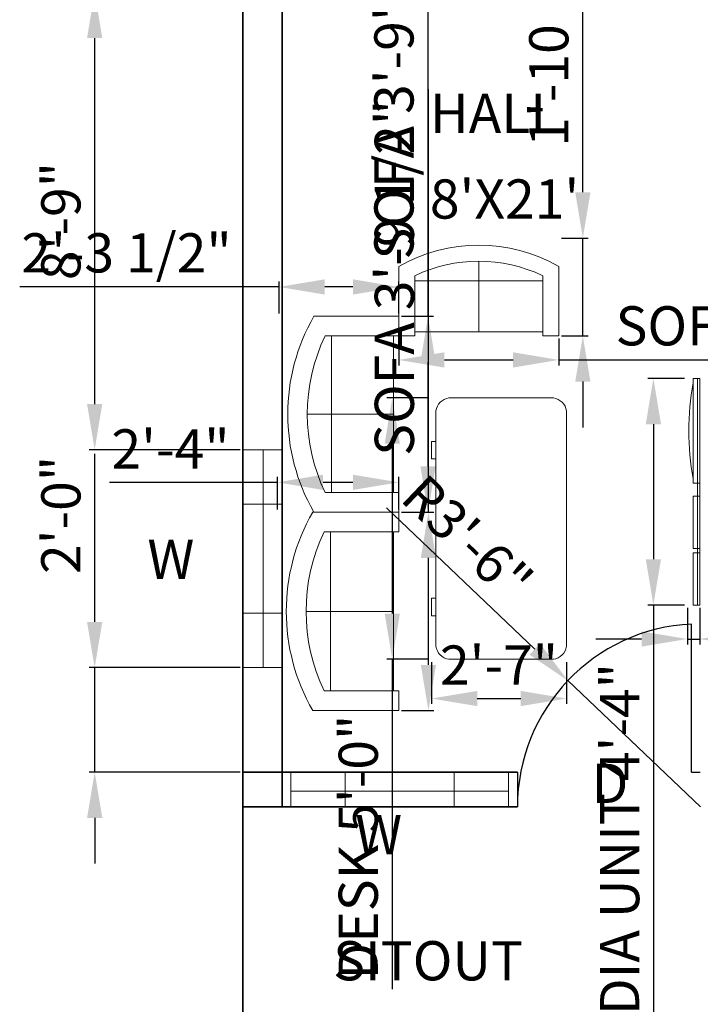
# Model space of a CAD drawing. Units: inches. Extents: x 1956 to 4770, y 1551 to 2596.
# Tile 3 of 10: x 2207 to 2363, y 1865 to 2091. Entities that reach past the tile are written whole.
import ezdxf

# ---------------------------------------------------------------- set-up
doc = ezdxf.new("R2010")
doc.units = ezdxf.units.IN
for name, color, linetype, lineweight in [('A-ANNO-DIMS', 2, 'Continuous', 18), ('A-ANNO-TEXT', 7, 'Continuous', 18), ('A-AREA-IDEN', 7, 'Continuous', 18), ('A-DOOR', 3, 'Continuous', 25), ('A-FURN', 8, 'Continuous', 18), ('A-GLAZ', 4, 'Continuous', 18), ('A-WALL', 7, 'Continuous', 35)]:
    doc.layers.add(name, color=color, linetype=linetype, lineweight=lineweight)
doc.styles.get("Standard").update_dxf_attribs({"font": 'arial.ttf'})
doc.dimstyles.new('ISO-25', dxfattribs={"dimtxt": 9, "dimasz": 10.5, "dimexe": 1.25, "dimexo": 0.625, "dimgap": 2, "dimtad": 1, "dimdec": 1, "dimlunit": 4, "dimtxsty": 'Standard', "dimcen": 2.5, "dimadec": 0, "dimazin": 0, "dimtfac": 1, "dimtdec": 1, "dimtmove": 0, "dimatfit": 3, "dimfxl": 1, "dimarcsym": 0})

# ---------------------------------------------------------------- blocks, each defined once
blk = doc.blocks.new('Sofa - Roundback Loveseat 5 ft.')
for p, q in [((0, -32.44198), (0, -5.99998)), ((-24, -33.99998), (-24, -11.46958)), ((24.00004, -33.99998), (24.00004, -11.46958)), ((-23.9998, -13.38178), (23.99986, -13.38178)), ((-24, -32.44198), (24.00004, -32.44198))]:
    blk.add_line(p, q)
for points in [[(-24, -33.99998), (-30, -33.99998), (-30, -7.99998)], [(30.00004, -7.99998), (30.00004, -33.99998), (24.00004, -33.99998)]]:
    blk.add_lwpolyline(points)
for centre, radius, start, end in [((0, -60.24998), 60.24998, 60.13715, 119.8628), ((0, -61.38438), 55.38444, 64.32083, 115.6792)]:
    blk.add_arc(centre, radius, start, end)
blk = doc.blocks.new('Desk - 30 x 60 in.')
for p, q in [((-26.999995, 0), (26.999995, 0)), ((-29.999995, -27), (-29.999995, -3)), ((29.999995, -3), (29.999995, -27)), ((26.999995, -30), (-26.999995, -30)), ((-20.000005, -30), (-20.000005, -31)), ((-20.000005, -31), (-16.000005, -31)), ((-16.000005, -31), (-16.000005, -30)), ((15.999995, -31), (15.999995, -30)), ((19.999995, -31), (15.999995, -31)), ((19.999995, -30), (19.999995, -31))]:
    blk.add_line(p, q)
for centre, start, end in [((-26.499995, -3.5), 98.1301, 171.8699), ((26.499995, -3.5), 8.130102, 81.8699), ((-26.499995, -26.5), 188.1301, 261.8699), ((26.499995, -26.5), 278.1301, 351.8699)]:
    blk.add_arc(centre, 3.535534, start, end)
blk = doc.blocks.new('Entertainment Center')
for p, q in [((-12, -20), (-12, -18.5)), ((40, -18.5), (-12, -18.5)), ((40, -19), (-12, -19)), ((12, -20), (-12, -20)), ((12, -18.5), (12, -20)), ((15, -20), (15, -18.5)), ((27, -20), (15, -20)), ((27, -18.5), (27, -20)), ((28, -20), (28, -18.5)), ((40, -20), (28, -20)), ((40, -18.5), (40, -20))]:
    blk.add_line(p, q)
blk.add_arc((0, 40), 61, 259.6111, 280.3889)
blk = doc.blocks.new('WIN-50IN-WALL9')
for p, q in [((0, 50), (9, 50)), ((4.6, 50), (4.6, 0)), ((0, 37.5), (9, 37.5)), ((9, 12.5), (0, 12.5)), ((9, 0), (1, 0)), ((0, 0), (9, 0))]:
    blk.add_line(p, q)
blk = doc.blocks.new('WIN-50IN-WALL8')
for p, q in [((0, 0), (0, 8)), ((12.5, 0), (12.5, 8)), ((37.5, 8), (37.5, 0)), ((50, 8), (50, 0)), ((0, 3.6), (50, 3.6))]:
    blk.add_line(p, q)
blk = doc.blocks.new('*D31')
at = {"layer": 'A-ANNO-DIMS', "color": 0, "lineweight": -2, "transparency": 16777216}
for p, q in [((2294, 2017.6), (2294, 2011.46)), ((2330.76, 2017.6), (2330.76, 2011.46)), ((2304.5, 2012.71), (2320.26, 2012.71)), ((2330.76, 2012.71), (2406.87, 2012.71))]:
    blk.add_line(p, q, dxfattribs=at)
at = {"layer": 'A-ANNO-DIMS', "color": 0, "transparency": 16777216}
for points in [[(2304.5, 2014.46), (2304.5, 2010.96), (2294, 2012.71)], [(2320.26, 2014.46), (2320.26, 2010.96), (2330.76, 2012.71)]]:
    blk.add_solid(points, dxfattribs=at)
at = {"layer": 'Defpoints', "color": 0, "transparency": 16777216}
for p in [(2294, 2018.23), (2330.76, 2018.23), (2330.76, 2012.71)]:
    blk.add_point(p, dxfattribs=at)
at = {"layer": 'A-ANNO-DIMS', "color": 0, "transparency": 16777216, "insert": (2374.07, 2019.37), "char_height": 9, "attachment_point": 5}
blk.add_mtext('SOFA 3\'-1"', dxfattribs=at)
blk = doc.blocks.new('*D32')
at = {"layer": 'A-ANNO-DIMS', "color": 0, "lineweight": -2, "transparency": 16777216}
for p, q in [((2336.28, 2051.19), (2336.28, 2116.73)), ((2331.39, 2040.69), (2337.53, 2040.69)), ((2336.28, 2018.23), (2336.28, 2040.69)), ((2331.39, 2018.23), (2337.53, 2018.23)), ((2336.28, 2007.73), (2336.28, 1997.23))]:
    blk.add_line(p, q, dxfattribs=at)
at = {"layer": 'A-ANNO-DIMS', "color": 0, "transparency": 16777216}
for points in [[(2334.53, 2051.19), (2338.03, 2051.19), (2336.28, 2040.69)], [(2334.53, 2007.73), (2338.03, 2007.73), (2336.28, 2018.23)]]:
    blk.add_solid(points, dxfattribs=at)
at = {"layer": 'Defpoints', "color": 0, "transparency": 16777216}
for p in [(2330.76, 2040.69), (2336.28, 2040.69), (2330.76, 2018.23)]:
    blk.add_point(p, dxfattribs=at)
at = {"layer": 'A-ANNO-DIMS', "color": 0, "transparency": 16777216, "insert": (2329.63, 2089.21), "char_height": 9, "attachment_point": 5, "rotation": 90}
blk.add_mtext('1\'-10 1/2"', dxfattribs=at)
blk = doc.blocks.new('*D33')
at = {"layer": 'A-ANNO-DIMS', "color": 0, "lineweight": -2, "transparency": 16777216}
for p, q in [((2300.83, 1977.77), (2300.83, 2074.85)), ((2294.63, 1977.77), (2302.08, 1977.77)), ((2300.83, 1942.72), (2300.83, 1967.27)), ((2294.63, 1932.22), (2302.08, 1932.22))]:
    blk.add_line(p, q, dxfattribs=at)
at = {"layer": 'A-ANNO-DIMS', "color": 0, "transparency": 16777216}
for points in [[(2299.08, 1967.27), (2302.58, 1967.27), (2300.83, 1977.77)], [(2299.08, 1942.72), (2302.58, 1942.72), (2300.83, 1932.22)]]:
    blk.add_solid(points, dxfattribs=at)
at = {"layer": 'Defpoints', "color": 0, "transparency": 16777216}
for p in [(2294, 1977.77), (2300.83, 1977.77), (2294, 1932.22)]:
    blk.add_point(p, dxfattribs=at)
at = {"layer": 'A-ANNO-DIMS', "color": 0, "transparency": 16777216, "insert": (2294.17, 2031.56), "char_height": 9, "attachment_point": 5, "rotation": 90}
blk.add_mtext('SOFA 3\'-9 1/2"', dxfattribs=at)
blk = doc.blocks.new('*D34')
at = {"layer": 'A-ANNO-DIMS', "color": 0, "lineweight": -2, "transparency": 16777216}
for p, q in [((2266.16, 1984.61), (2227.58, 1984.61)), ((2266.16, 1978.4), (2266.16, 1985.86)), ((2283.5, 1984.61), (2276.66, 1984.61)), ((2294, 1978.4), (2294, 1985.86))]:
    blk.add_line(p, q, dxfattribs=at)
at = {"layer": 'A-ANNO-DIMS', "color": 0, "transparency": 16777216}
for points in [[(2276.66, 1986.36), (2276.66, 1982.86), (2266.16, 1984.61)], [(2283.5, 1986.36), (2283.5, 1982.86), (2294, 1984.61)]]:
    blk.add_solid(points, dxfattribs=at)
at = {"layer": 'Defpoints', "color": 0, "transparency": 16777216}
for p in [(2266.16, 1984.61), (2266.16, 1977.77), (2294, 1977.77)]:
    blk.add_point(p, dxfattribs=at)
at = {"layer": 'A-ANNO-DIMS', "color": 0, "transparency": 16777216, "insert": (2241.62, 1991.12), "char_height": 9, "attachment_point": 5}
blk.add_mtext('2\'-4"', dxfattribs=at)
blk = doc.blocks.new('*D35')
at = {"layer": 'A-ANNO-DIMS', "color": 0, "lineweight": -2, "transparency": 16777216}
for p, q in [((2300.74, 2022.72), (2300.74, 2098.83)), ((2294.63, 2022.72), (2301.99, 2022.72)), ((2300.74, 1988.27), (2300.74, 2012.22)), ((2294.63, 1977.77), (2301.99, 1977.77))]:
    blk.add_line(p, q, dxfattribs=at)
at = {"layer": 'A-ANNO-DIMS', "color": 0, "transparency": 16777216}
for points in [[(2298.99, 2012.22), (2302.49, 2012.22), (2300.74, 2022.72)], [(2298.99, 1988.27), (2302.49, 1988.27), (2300.74, 1977.77)]]:
    blk.add_solid(points, dxfattribs=at)
at = {"layer": 'Defpoints', "color": 0, "transparency": 16777216}
for p in [(2294, 2022.72), (2300.74, 2022.72), (2294, 1977.77)]:
    blk.add_point(p, dxfattribs=at)
at = {"layer": 'A-ANNO-DIMS', "color": 0, "transparency": 16777216, "insert": (2294.08, 2066.02), "char_height": 9, "attachment_point": 5, "rotation": 90}
blk.add_mtext('SOFA 3\'-9"', dxfattribs=at)
blk = doc.blocks.new('*D36')
at = {"layer": 'A-ANNO-DIMS', "color": 0, "lineweight": -2, "transparency": 16777216}
for p, q in [((2266.53, 2023.35), (2266.53, 2030.71)), ((2294, 2023.35), (2294, 2030.71)), ((2266.53, 2029.46), (2206.98, 2029.46)), ((2283.5, 2029.46), (2277.03, 2029.46))]:
    blk.add_line(p, q, dxfattribs=at)
at = {"layer": 'A-ANNO-DIMS', "color": 0, "transparency": 16777216}
for points in [[(2277.03, 2031.21), (2277.03, 2027.71), (2266.53, 2029.46)], [(2283.5, 2031.21), (2283.5, 2027.71), (2294, 2029.46)]]:
    blk.add_solid(points, dxfattribs=at)
at = {"layer": 'Defpoints', "color": 0, "transparency": 16777216}
for p in [(2266.53, 2029.46), (2266.53, 2022.72), (2294, 2022.72)]:
    blk.add_point(p, dxfattribs=at)
at = {"layer": 'A-ANNO-DIMS', "color": 0, "transparency": 16777216, "insert": (2231.51, 2036.12), "char_height": 9, "attachment_point": 5}
blk.add_mtext('2\'-3 1/2"', dxfattribs=at)
blk = doc.blocks.new('*D59')
at = {"layer": 'A-ANNO-DIMS', "color": 0, "lineweight": -2, "transparency": 16777216}
for p, q in [((2300.91, 2003.99), (2291.28, 2003.99)), ((2292.53, 1993.49), (2292.53, 1954.49)), ((2300.91, 1943.99), (2291.28, 1943.99)), ((2292.53, 1943.99), (2292.53, 1868.28))]:
    blk.add_line(p, q, dxfattribs=at)
at = {"layer": 'A-ANNO-DIMS', "color": 0, "transparency": 16777216}
for points in [[(2290.78, 1993.49), (2294.28, 1993.49), (2292.53, 2003.99)], [(2290.78, 1954.49), (2294.28, 1954.49), (2292.53, 1943.99)]]:
    blk.add_solid(points, dxfattribs=at)
at = {"layer": 'Defpoints', "color": 0, "transparency": 16777216}
for p in [(2301.53, 2003.99), (2292.53, 1943.99), (2301.53, 1943.99)]:
    blk.add_point(p, dxfattribs=at)
at = {"layer": 'A-ANNO-DIMS', "color": 0, "transparency": 16777216, "insert": (2285.88, 1900.88), "char_height": 9, "attachment_point": 5, "rotation": 90}
blk.add_mtext('DESK 5\'-0"', dxfattribs=at)
blk = doc.blocks.new('*D60')
at = {"layer": 'A-ANNO-DIMS', "color": 0, "lineweight": -2, "transparency": 16777216}
for p, q in [((2301.53, 1943.36), (2301.53, 1933.74)), ((2332.53, 1943.36), (2332.53, 1933.74)), ((2312.03, 1934.99), (2322.03, 1934.99))]:
    blk.add_line(p, q, dxfattribs=at)
at = {"layer": 'A-ANNO-DIMS', "color": 0, "transparency": 16777216}
for points in [[(2312.03, 1936.74), (2312.03, 1933.24), (2301.53, 1934.99)], [(2322.03, 1936.74), (2322.03, 1933.24), (2332.53, 1934.99)]]:
    blk.add_solid(points, dxfattribs=at)
at = {"layer": 'Defpoints', "color": 0, "transparency": 16777216}
for p in [(2301.53, 1943.99), (2332.53, 1943.99), (2332.53, 1934.99)]:
    blk.add_point(p, dxfattribs=at)
at = {"layer": 'A-ANNO-DIMS', "color": 0, "transparency": 16777216, "insert": (2317.03, 1941.5), "char_height": 9, "attachment_point": 5}
blk.add_mtext('2\'-7"', dxfattribs=at)
blk = doc.blocks.new('*D61')
at = {"layer": 'A-ANNO-DIMS', "color": 0, "lineweight": -2, "transparency": 16777216}
for p, q in [((2359.65, 2008.45), (2351.23, 2008.45)), ((2352.48, 1997.95), (2352.48, 1966.95)), ((2359.65, 1956.45), (2351.23, 1956.45)), ((2352.48, 1956.45), (2352.48, 1842.3))]:
    blk.add_line(p, q, dxfattribs=at)
at = {"layer": 'A-ANNO-DIMS', "color": 0, "transparency": 16777216}
for points in [[(2350.73, 1997.95), (2354.23, 1997.95), (2352.48, 2008.45)], [(2350.73, 1966.95), (2354.23, 1966.95), (2352.48, 1956.45)]]:
    blk.add_solid(points, dxfattribs=at)
at = {"layer": 'Defpoints', "color": 0, "transparency": 16777216}
for p in [(2360.28, 2008.45), (2352.48, 1956.45), (2360.28, 1956.45)]:
    blk.add_point(p, dxfattribs=at)
at = {"layer": 'A-ANNO-DIMS', "color": 0, "transparency": 16777216, "insert": (2345.9, 1894.13), "char_height": 9, "attachment_point": 5, "rotation": 90}
blk.add_mtext('MEDIA UNIT 4\'-4"', dxfattribs=at)
blk = doc.blocks.new('*D62')
at = {"layer": 'A-ANNO-DIMS', "color": 0, "lineweight": -2, "transparency": 16777216}
for p, q in [((2360.28, 1955.83), (2360.28, 1947.4)), ((2363.11, 1955.83), (2363.11, 1947.4)), ((2349.78, 1948.65), (2339.28, 1948.65)), ((2360.28, 1948.65), (2363.11, 1948.65)), ((2373.61, 1948.65), (2412.03, 1948.65))]:
    blk.add_line(p, q, dxfattribs=at)
at = {"layer": 'A-ANNO-DIMS', "color": 0, "transparency": 16777216}
for points in [[(2349.78, 1950.4), (2349.78, 1946.9), (2360.28, 1948.65)], [(2373.61, 1950.4), (2373.61, 1946.9), (2363.11, 1948.65)]]:
    blk.add_solid(points, dxfattribs=at)
at = {"layer": 'Defpoints', "color": 0, "transparency": 16777216}
for p in [(2360.28, 1956.45), (2363.11, 1956.45), (2363.11, 1948.65)]:
    blk.add_point(p, dxfattribs=at)
at = {"layer": 'A-ANNO-DIMS', "color": 0, "transparency": 16777216, "insert": (2398.07, 1955.25), "char_height": 9, "attachment_point": 5}
blk.add_mtext('0\'-3"', dxfattribs=at)
blk = doc.blocks.new('*D65')
at = {"layer": 'A-ANNO-DIMS', "color": 0, "lineweight": -2, "transparency": 16777216}
for p, q in [((2224.2, 1952.59), (2224.2, 1991.16)), ((2257.63, 1942.09), (2222.95, 1942.09)), ((2224.2, 1918.09), (2224.2, 1942.09)), ((2257.63, 1918.09), (2222.95, 1918.09)), ((2224.2, 1907.59), (2224.2, 1897.09))]:
    blk.add_line(p, q, dxfattribs=at)
at = {"layer": 'A-ANNO-DIMS', "color": 0, "transparency": 16777216}
for points in [[(2222.45, 1952.59), (2225.95, 1952.59), (2224.2, 1942.09)], [(2222.45, 1907.59), (2225.95, 1907.59), (2224.2, 1918.09)]]:
    blk.add_solid(points, dxfattribs=at)
at = {"layer": 'Defpoints', "color": 0, "transparency": 16777216}
for p in [(2224.2, 1942.09), (2258.25, 1942.09), (2258.25, 1918.09)]:
    blk.add_point(p, dxfattribs=at)
at = {"layer": 'A-ANNO-DIMS', "color": 0, "transparency": 16777216, "insert": (2217.61, 1977.13), "char_height": 9, "attachment_point": 5, "rotation": 90}
blk.add_mtext('2\'-0"', dxfattribs=at)
blk = doc.blocks.new('*D66')
at = {"layer": 'A-ANNO-DIMS', "color": 0, "lineweight": -2, "transparency": 16777216}
for p, q in [((2257.63, 2097.09), (2222.95, 2097.09)), ((2224.2, 2002.59), (2224.2, 2086.59)), ((2257.63, 1992.09), (2222.95, 1992.09))]:
    blk.add_line(p, q, dxfattribs=at)
at = {"layer": 'A-ANNO-DIMS', "color": 0, "transparency": 16777216}
for points in [[(2222.45, 2086.59), (2225.95, 2086.59), (2224.2, 2097.09)], [(2222.45, 2002.59), (2225.95, 2002.59), (2224.2, 1992.09)]]:
    blk.add_solid(points, dxfattribs=at)
at = {"layer": 'Defpoints', "color": 0, "transparency": 16777216}
for p in [(2224.2, 2097.09), (2258.25, 2097.09), (2258.25, 1992.09)]:
    blk.add_point(p, dxfattribs=at)
at = {"layer": 'A-ANNO-DIMS', "color": 0, "transparency": 16777216, "insert": (2217.61, 2044.59), "char_height": 9, "attachment_point": 5, "rotation": 90}
blk.add_mtext('8\'-9"', dxfattribs=at)
blk = doc.blocks.new('*D104')
at = {"layer": 'A-ANNO-DIMS', "color": 0, "lineweight": -2, "transparency": 16777216}
for p, q in [((2291.19, 1978.77), (2325.25, 1946.33)), ((2363.3, 1910.09), (2332.85, 1939.09))]:
    blk.add_line(p, q, dxfattribs=at)
at = {"layer": 'A-ANNO-DIMS', "color": 0, "transparency": 16777216}
blk.add_solid([(2326.46, 1947.59), (2324.04, 1945.06), (2332.85, 1939.09)], dxfattribs=at)
at = {"layer": 'Defpoints', "color": 0, "transparency": 16777216}
for p in [(2332.85, 1939.09), (2363.3, 1910.09)]:
    blk.add_point(p, dxfattribs=at)
at = {"layer": 'A-ANNO-DIMS', "color": 0, "transparency": 16777216, "insert": (2308.97, 1970.95), "char_height": 9, "attachment_point": 5, "rotation": 316.3978}
blk.add_mtext('R3\'-6"', dxfattribs=at)

msp = doc.modelspace()

# ---------------------------------------------------------------- linework, layer by layer
at = {"layer": 'A-DOOR'}
for p, q in [((2361.25, 1918.09), (2361.25, 1952.09)), ((2321.25, 1918.09), (2321.25, 1910.09)), ((2361.25, 1918.09), (2363.25, 1918.09))]:
    msp.add_line(p, q, dxfattribs=at)
msp.add_arc((2363.3, 1910.09), 42.05, 92.7944, 180, dxfattribs=at)
at = {"layer": 'A-WALL'}
for p, q in [((2258.25, 1757.09), (2258.25, 2309.09)), ((2267.25, 1910.09), (2267.25, 2309.09)), ((2258.25, 1918.09), (2321.25, 1918.09)), ((2258.25, 1910.09), (2267.25, 1910.09)), ((2321.25, 1910.09), (2267.25, 1910.09))]:
    msp.add_line(p, q, dxfattribs=at)

# ---------------------------------------------------------------- block references
at = {"layer": 'A-FURN', "xscale": 0.6127256065677673, "yscale": 0.6127256065677673, "zscale": 0.6127256065677673}
msp.add_blockref('Sofa - Roundback Loveseat 5 ft.', (2312.38, 2039.06), dxfattribs=at)
at = {"layer": 'A-FURN', "rotation": 90}
for p, xscale, yscale, zscale in [((2268.53, 2000.25), 0.7491442860294625, 0.7491442860294625, 0.7491442860294625), ((2268.19, 1955), 0.7592175691499663, 0.7592175691499663, 0.7592175691499663)]:
    msp.add_blockref('Sofa - Roundback Loveseat 5 ft.', p, dxfattribs=dict(at, xscale=xscale, yscale=yscale, zscale=zscale))
at = {"layer": 'A-FURN', "rotation": 270}
for name, p in [('Entertainment Center', (2381.61, 1996.45)), ('Desk - 30 x 60 in.', (2332.53, 1973.99))]:
    msp.add_blockref(name, p, dxfattribs=at)
at = {"layer": 'A-GLAZ'}
for name, p in [('WIN-50IN-WALL9', (2258.25, 1942.09)), ('WIN-50IN-WALL8', (2269.25, 1910.09))]:
    msp.add_blockref(name, p, dxfattribs=at)

# ---------------------------------------------------------------- texts
at = {"layer": 'A-ANNO-TEXT'}
for s, p in [('         W ', (2211.55, 1962.46)), ('D', (2338.28, 1911.01)), ('         W ', (2259.26, 1899.26))]:
    msp.add_text(s, height=9, dxfattribs=at).set_placement(p)
at = {"layer": 'A-AREA-IDEN'}
for s, p in [('  HALL', (2295.66, 2064.8)), ("  8'X21'", (2295.66, 2045.15)), (' SITOUT ', (2276.21, 1870.29))]:
    msp.add_text(s, height=9, dxfattribs=at).set_placement(p)

# ---------------------------------------------------------------- dimensions: what is measured, and where the dimension line sits
at = {"layer": 'A-ANNO-DIMS'}
for base, p1, p2, angle, picture, middle in [((2336.28, 2040.69), (2330.76, 2018.23), (2330.76, 2040.69), 90, '*D32', (2329.63, 2089.21)), ((2224.2, 2097.09), (2258.25, 1992.09), (2258.25, 2097.09), 90, '*D66', (2217.61, 2044.59)), ((2266.53, 2029.46), (2294, 2022.72), (2266.53, 2022.72), 180, '*D36', (2231.51, 2036.12)), ((2266.16, 1984.61), (2294, 1977.77), (2266.16, 1977.77), 180, '*D34', (2241.62, 1991.12)), ((2224.2, 1942.09), (2258.25, 1918.09), (2258.25, 1942.09), 90, '*D65', (2217.61, 1977.13))]:
    dim = msp.add_linear_dim(base=base, p1=p1, p2=p2, angle=angle, dimstyle='ISO-25', override={"dimdec": 1, "dimlfac": 1, "dimrnd": 0, "dimzin": 1, "dimdsep": 46, "dimlunit": 4, "dimfrac": 2}, dxfattribs=at)
    dim.commit()
    dim.dimension.update_dxf_attribs({"geometry": picture, "text_midpoint": middle})
for base, p1, p2, angle, text, picture, middle in [((2300.7428, 2022.7213), (2294.0005, 1977.7726), (2294.0005, 2022.7213), 90, 'SOFA <>', '*D35', (2294.0832, 2066.0245)), ((2300.8335, 1977.7726), (2294.0005, 1932.2195), (2294.0005, 1977.7726), 90, 'SOFA <>', '*D33', (2294.1739, 2031.5615)), ((2352.48, 1956.45), (2360.28, 2008.45), (2360.28, 1956.45), 270, 'MEDIA UNIT <>', '*D61', (2345.9, 1894.13)), ((2292.53, 1943.99), (2301.53, 2003.99), (2301.53, 1943.99), 270, 'DESK <>', '*D59', (2285.88, 1900.88))]:
    dim = msp.add_linear_dim(base=base, p1=p1, p2=p2, angle=angle, text=text, dimstyle='ISO-25', override={"dimdec": 1, "dimlfac": 1, "dimrnd": 0, "dimzin": 1, "dimdsep": 46, "dimlunit": 4, "dimfrac": 2}, dxfattribs=at)
    dim.commit()
    dim.dimension.update_dxf_attribs({"geometry": picture, "text_midpoint": middle})
dim = msp.add_linear_dim(base=(2330.76, 2012.71), p1=(2294, 2018.23), p2=(2330.76, 2018.23), text='SOFA <>', dimstyle='ISO-25', override={"dimdec": 1, "dimlfac": 1, "dimrnd": 0, "dimzin": 1, "dimdsep": 46, "dimlunit": 4, "dimfrac": 2}, dxfattribs=at)
dim.commit()
dim.dimension.update_dxf_attribs({"geometry": '*D31', "text_midpoint": (2374.07, 2019.37)})
dim = msp.add_radius_dim(center=(2363.30339, 1910.08628), mpoint=(2332.85306, 1939.08594), dimstyle='ISO-25', override={"dimdec": 1, "dimlfac": 1, "dimrnd": 0, "dimzin": 1, "dimdsep": 46, "dimlunit": 4, "dimfrac": 2}, dxfattribs=at)
dim.commit()
dim.dimension.update_dxf_attribs({"geometry": '*D104', "text_midpoint": (2308.96721, 1970.9456)})
for base, p1, p2, picture, middle in [((2363.11, 1948.65), (2360.28, 1956.45), (2363.11, 1956.45), '*D62', (2398.07, 1955.25)), ((2332.53, 1934.99), (2301.53, 1943.99), (2332.53, 1943.99), '*D60', (2317.03, 1941.5))]:
    dim = msp.add_linear_dim(base=base, p1=p1, p2=p2, dimstyle='ISO-25', override={"dimdec": 1, "dimlfac": 1, "dimrnd": 0, "dimzin": 1, "dimdsep": 46, "dimlunit": 4, "dimfrac": 2}, dxfattribs=at)
    dim.commit()
    dim.dimension.update_dxf_attribs({"geometry": picture, "text_midpoint": middle})

doc.saveas('drawing.dxf')
